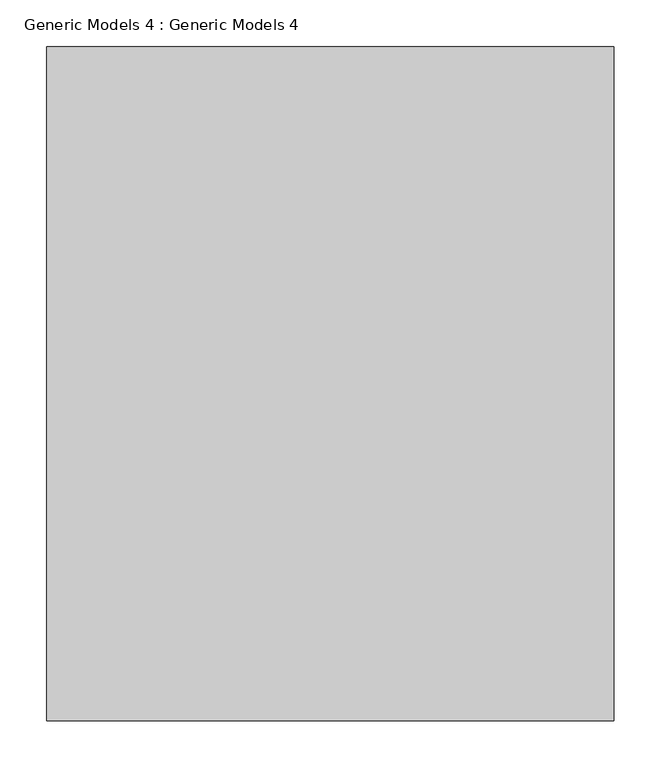
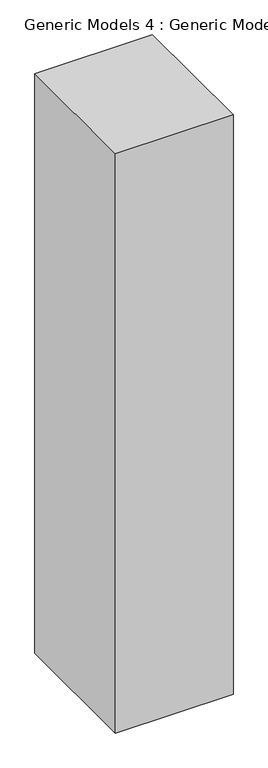
"""IFC4 building model written with IfcOpenShell, lengths in millimetres: proxy geometry, Generic Models 4 : Generic Models 4."""

from ifc_helpers import new_model, si_unit, frame, origin, place, context, project, spatial, polyline, outline, extrude, source, transform, mapped, element, save


def generic_models_4_generic_models_4_b7bd3587(model_context):
    return source(origin(), model_context, "Body", "SweptSolid", [
        extrude(outline(polyline([(-16209.27956, -4902.7088252), (-16818.87956, -4902.7088252), (-16818.87956, -4178.8088252), (-16209.27956, -4178.8088252), (-16209.27956, -4902.7088252)])), frame((0.0, 0.0, 4348.8306813), z_axis=(0.0, 0.0, 1.0), x_axis=(1.0, 0.0, 0.0)), (0.0, 0.0, 1.0), 3175.9193187),
    ])


if __name__ == "__main__":
    model = new_model("IFC4")
    model_context = context("Model", 3, world=origin())
    ifc_project = project(units=[si_unit("LENGTHUNIT", "METRE", prefix="MILLI")], contexts=[model_context])
    site = spatial("IfcSite", under=ifc_project)
    building = spatial("IfcBuilding", under=site)
    placement = place(None, origin())
    generic_models_4_generic_models_4_shape = generic_models_4_generic_models_4_b7bd3587(model_context)
    element("IfcBuildingElementProxy", 1, Name="Generic Models 4 : Generic Models 4", ObjectType="Generic Models 4 : Generic Models 4", at=placement, inside=building, context=model_context, shape_type="MappedRepresentation", body=[
        mapped(generic_models_4_generic_models_4_shape, transform((0.0, 0.0, 0.0), x_axis=(1.0, 0.0, 0.0), y_axis=(0.0, 1.0, 0.0), z_axis=(0.0, 0.0, 1.0))),
    ])
    save(model, "model.ifc")
